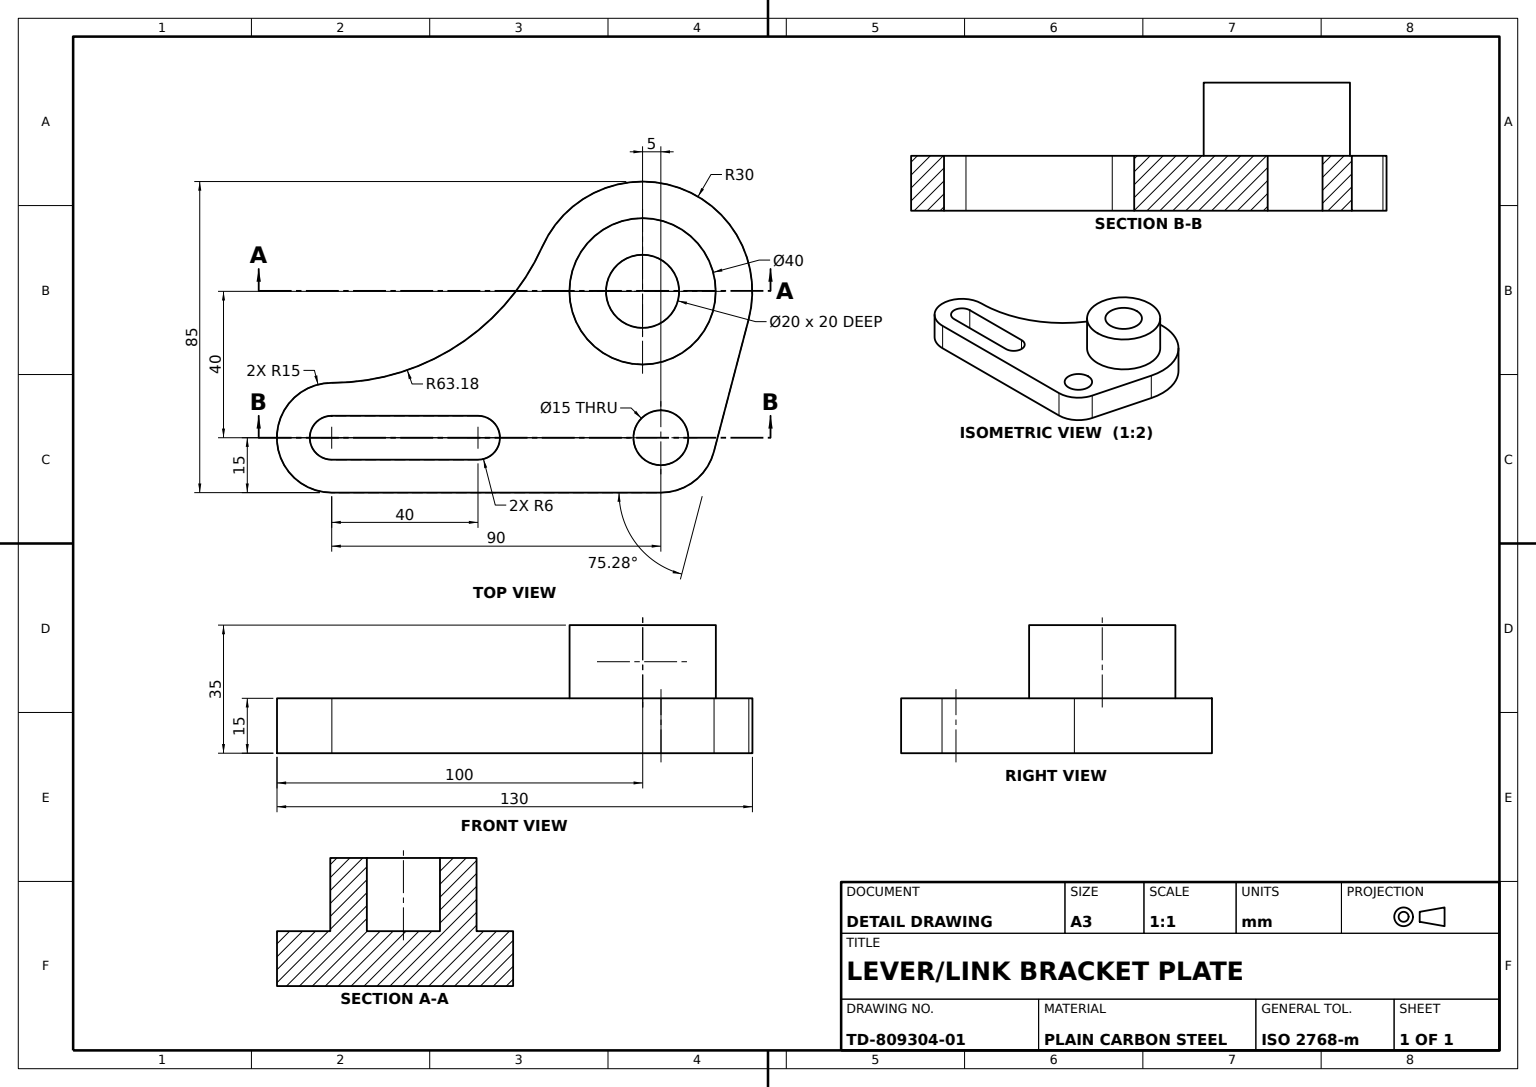
SolidWorks part; units mm, degrees
material "Plain Carbon Steel"
ref_plane "Front Plane" through (0, 0, 0) normal (0, 0, 1) x (1, 0, 0)
ref_plane "Top Plane" through (0, 0, 0) normal (0, 1, 0) x (1, 0, 0)
ref_plane "Right Plane" through (0, 0, 0) normal (1, 0, 0) x (0, 0, -1)
sketch "Link Plate Profile" plane through (0, 0, 0) normal (0, 1, 0) x (1, 0, 0)
  line L0 (114.0153, 32.3769) -> (104.5077, -3.8115)
  line L1 (0, -15) -> (90, -15)
  arc A0 (0, 15) -> (0, -15) centre (0, 0) ccw
  arc A1 (90, -15) -> (104.5077, -3.8115) centre (90, 0) ccw
  arc A2 (114.0153, 32.3769) -> (57.6341, 52.2927) centre (85, 40) ccw
  arc A3 (0, 15) -> (57.6341, 52.2927) centre (0, 78.1818) ccw
  dimension "D1" = 90
  dimension "D4" = 30
  dimension "D5" = 30
  dimension "D6" = 60
  dimension "D2" = 5
  dimension "D3" = 40
extrude "Link Plate 15mm" add sketch "Link Plate Profile" along normal blind 15
sketch "Slot Profile" plane through (0, 15, 0) normal (0, 1, 0) x (1, 0, 0)
  line L0 (0, 0) -> (40, 0) construction
  line L1 (0, 6) -> (40, 6)
  line L2 (0, -6) -> (40, -6)
  arc A0 (0, 6) -> (0, -6) centre (0, 0) ccw
  arc A1 (40, -6) -> (40, 6) centre (40, 0) ccw
  point P3 (20, 0)
  dimension "D2" = 6
  dimension "D1" = 40
extrude "Slot Cut" cut sketch "Slot Profile" against normal through all
sketch "Through Hole Profile" plane through (0, 15, 0) normal (0, 1, 0) x (1, 0, 0)
  circle A0 centre (90, 0) radius 7.5
  dimension "D1" = 15
extrude "Through Hole Cut" cut sketch "Through Hole Profile" against normal blind 15
sketch "Pivot Boss Profile Ø40-Ø20" plane through (0, 15, 0) normal (0, 1, 0) x (1, 0, 0)
  circle A0 centre (85, 40) radius 20
  circle A1 centre (85, 40) radius 10
  dimension "D1" = 40
  dimension "D2" = 20
extrude "Pivot Boss Ø40" add sketch "Pivot Boss Profile Ø40-Ø20" along normal blind 20
